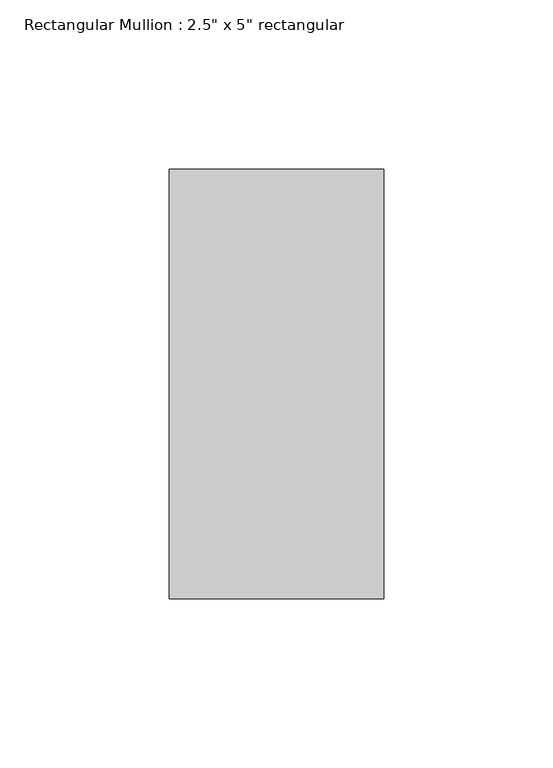
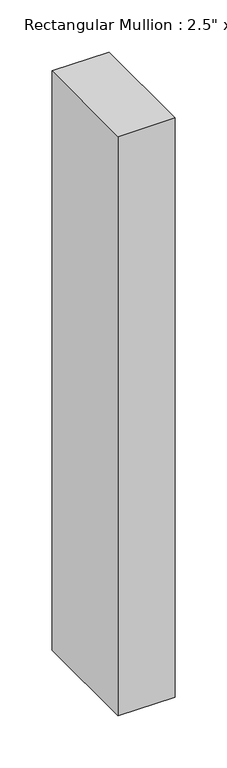
"""IFC4 building model written with IfcOpenShell, lengths in millimetres: member geometry."""

from ifc_helpers import new_model, si_unit, frame, origin, place, context, project, spatial, polyline, outline, extrude, source, transform, mapped, element, save


def member_3cc62806(model_context):
    return source(origin(), model_context, "Body", "SweptSolid", [
        extrude(outline(polyline([(0.0, 63.5), (0.0, -63.5), (-63.5, -63.5), (-63.5, 63.5), (0.0, 63.5)])), frame((0.0, 0.0, -680.0388769), z_axis=(0.0, 0.0, 1.0), x_axis=(1.0, 0.0, 0.0)), (0.0, 0.0, 1.0), 680.0388769),
    ])


if __name__ == "__main__":
    model = new_model("IFC4")
    model_context = context("Model", 3, world=origin())
    ifc_project = project(units=[si_unit("LENGTHUNIT", "METRE", prefix="MILLI")], contexts=[model_context])
    site = spatial("IfcSite", under=ifc_project)
    building = spatial("IfcBuilding", under=site)
    placement = place(None, origin())
    member_shape = member_3cc62806(model_context)
    element("IfcMember", 1, ObjectType="Rectangular Mullion : 2.5\" x 5\" rectangular", at=placement, inside=building, context=model_context, shape_type="MappedRepresentation", body=[
        mapped(member_shape, transform((0.0, 0.0, 0.0), x_axis=(1.0, 0.0, 0.0), y_axis=(0.0, 1.0, 0.0), z_axis=(0.0, 0.0, 1.0))),
    ])
    save(model, "model.ifc")

# Revit data of these elements
# Type "Rectangular Mullion : 2.5\" x 5\" rectangular"
#   built-in parameter 1007304 = 0.416667 (stored number, unit not read)
#   built-in parameter 1007301 = 0.104167 (stored number, unit not read)
#   built-in parameter 1007300 = 0.104167 (stored number, unit not read)
# Element 1 (IfcMember, "Rectangular Mullion : 2.5\" x 5\" rectangular")
#   Materials on its faces: "Aluminum"
# Materials
#   "Aluminum": class "Metal", colour RGB 247 247 247, transparency 0, Description = "Aluminum 6061", Cost = 0
